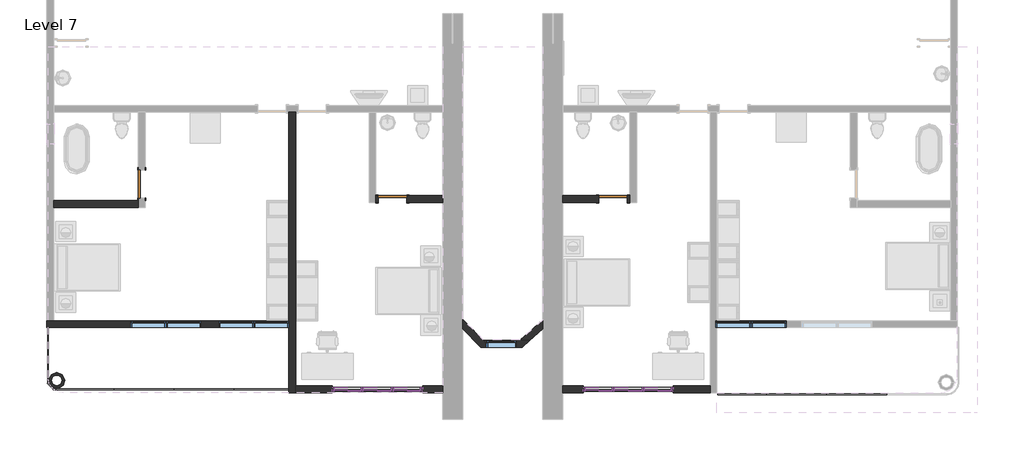
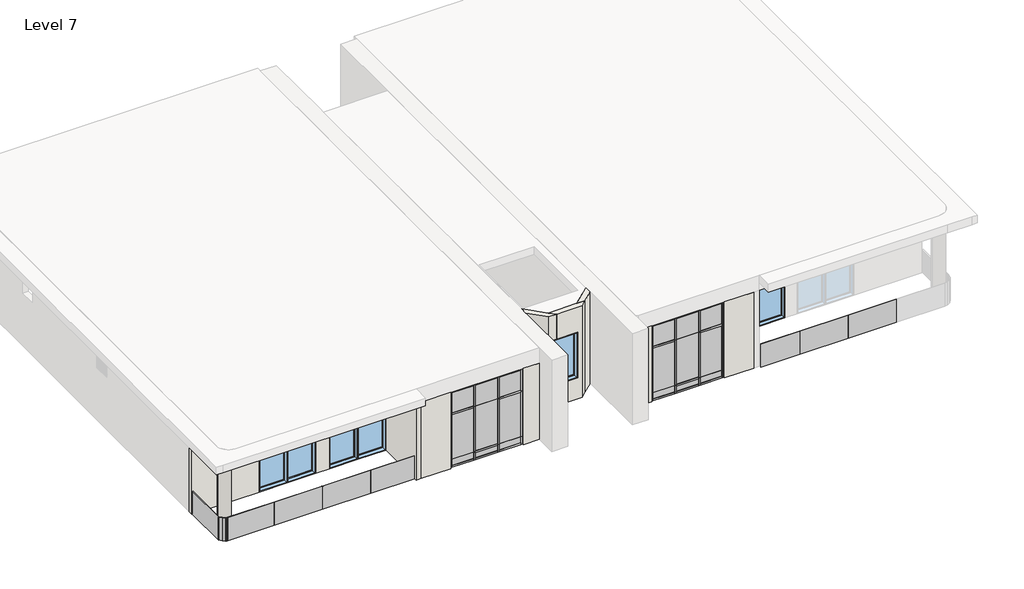
# One storey, part 1 of 3: 42 members, 30 plates, 14 walls, 7 windows, 3 doors.
"""IFC4 building model written with IfcOpenShell, lengths in millimetres."""

from ifc_helpers import new_model, si_unit, point, frame, frame_2d, origin, place, context, project, spatial, polyline, circle_curve, trimmed, segment, composite_curve, outline, extrude, faceted_brep, transform, mapped, element, save
from components import door_2703ae13, door_10fd3a06, member_c17f1be2, member_ad567e07, member_d2e7e466, member_7db1855a, member_75d1e245, member_d60e8053, member_3c3dc66a, member_2fae0574, member_410c6227, member_73c23c35, system_panel_glazed_38d54ecf, system_panel_glazed_fbb6c980, system_panel_glazed_4137532c, system_panel_glazed_6230de04, system_panel_glazed_a79f7f85, system_panel_glazed_9a5ea490, system_panel_glazed_95be5de7, system_panel_glazed_1e00a1c5, system_panel_glazed_ffe51582, system_panel_glazed_8f95e3f6, system_panel_glazed_836907cd, system_panel_glazed_688a65a2, system_panel_glazed_c1a1c740, system_panel_glazed_22bcd51f, window_9a779fa2, window_1a213a25

model = new_model("IFC4")

# Units and contexts
model_context = context("Model", 3, world=origin())
ifc_project = project(units=[si_unit("LENGTHUNIT", "METRE", prefix="MILLI")], contexts=[model_context])

# Site, building, storey
site = spatial("IfcSite", under=ifc_project)
building = spatial("IfcBuilding", under=site)
storey = spatial("IfcBuildingStorey", under=building, Name="Level 7", Elevation=21945.6)

# Doors
placement = place(None, origin())
door_shape = door_2703ae13(model_context)
element("IfcDoor", 1, ObjectType="Door-Single-Panel.0001 : 34\" x 80\"", at=placement, inside=storey, context=model_context, shape_type="MappedRepresentation", body=[
    mapped(door_shape, transform((-15759.6487704, -441.9241442, 21945.6), x_axis=(0.0, -1.0, 0.0), y_axis=(1.0, 0.0, 0.0), z_axis=(0.0, 0.0, 1.0))),
])
element("IfcDoor", 2, ObjectType="Door-Single-Panel.0001 : 34\" x 80\"", at=placement, inside=storey, context=model_context, shape_type="MappedRepresentation", body=[
    mapped(door_shape, transform((-8139.6487704, -899.1241442, 21945.6), x_axis=(-1.0, 0.0, 0.0), y_axis=(0.0, -1.0, 0.0), z_axis=(0.0, 0.0, 1.0))),
])
door_2_shape = door_10fd3a06(model_context)
element("IfcDoor", 3, ObjectType="Door-Single-Panel.0001 : 34\" x 80\"", at=placement, inside=storey, context=model_context, shape_type="MappedRepresentation", body=[
    mapped(door_2_shape, transform((-1434.0487704, -899.1241442, 21945.6), x_axis=(1.0, 0.0, 0.0), y_axis=(0.0, 1.0, 0.0), z_axis=(0.0, 0.0, 1.0))),
])

# Members
member_shape = member_c17f1be2(model_context)
element("IfcMember", 4, ObjectType="Rectangular Mullion : 2.5\" x 5\" rectangular", at=placement, inside=storey, context=model_context, shape_type="MappedRepresentation", body=[
    mapped(member_shape, transform((-9904.9487704, -6690.3241442, 24993.6), x_axis=(0.0, 0.0, 1.0), y_axis=(0.0, 1.0, 0.0), z_axis=(-1.0, 0.0, 0.0))),
])
element("IfcMember", 5, ObjectType="Rectangular Mullion : 2.5\" x 5\" rectangular", at=placement, inside=storey, context=model_context, shape_type="MappedRepresentation", body=[
    mapped(member_shape, transform((-8107.8987704, -6690.3241442, 24993.6), x_axis=(0.0, 0.0, 1.0), y_axis=(0.0, 1.0, 0.0), z_axis=(-1.0, 0.0, 0.0))),
])
element("IfcMember", 6, ObjectType="Rectangular Mullion : 2.5\" x 5\" rectangular", at=placement, inside=storey, context=model_context, shape_type="MappedRepresentation", body=[
    mapped(member_shape, transform((-2284.9487704, -6690.3241442, 24993.6), x_axis=(0.0, 0.0, 1.0), y_axis=(0.0, 1.0, 0.0), z_axis=(-1.0, 0.0, 0.0))),
])
element("IfcMember", 7, ObjectType="Rectangular Mullion : 2.5\" x 5\" rectangular", at=placement, inside=storey, context=model_context, shape_type="MappedRepresentation", body=[
    mapped(member_shape, transform((-487.8987704, -6690.3241442, 24993.6), x_axis=(0.0, 0.0, 1.0), y_axis=(0.0, 1.0, 0.0), z_axis=(-1.0, 0.0, 0.0))),
])
element("IfcMember", 8, ObjectType="Rectangular Mullion : 2.5\" x 5\" rectangular", at=placement, inside=storey, context=model_context, shape_type="MappedRepresentation", body=[
    mapped(member_shape, transform((-7288.7487704, -6690.3241442, 21945.6), x_axis=(0.0, 0.0, -1.0), y_axis=(0.0, 1.0, 0.0), z_axis=(1.0, 0.0, 0.0))),
])
element("IfcMember", 9, ObjectType="Rectangular Mullion : 2.5\" x 5\" rectangular", at=placement, inside=storey, context=model_context, shape_type="MappedRepresentation", body=[
    mapped(member_shape, transform((-9085.7987704, -6690.3241442, 21945.6), x_axis=(0.0, 0.0, -1.0), y_axis=(0.0, 1.0, 0.0), z_axis=(1.0, 0.0, 0.0))),
])
element("IfcMember", 10, ObjectType="Rectangular Mullion : 2.5\" x 5\" rectangular", at=placement, inside=storey, context=model_context, shape_type="MappedRepresentation", body=[
    mapped(member_shape, transform((331.2512296, -6690.3241442, 21945.6), x_axis=(0.0, 0.0, -1.0), y_axis=(0.0, 1.0, 0.0), z_axis=(1.0, 0.0, 0.0))),
])
element("IfcMember", 11, ObjectType="Rectangular Mullion : 2.5\" x 5\" rectangular", at=placement, inside=storey, context=model_context, shape_type="MappedRepresentation", body=[
    mapped(member_shape, transform((-1465.7987704, -6690.3241442, 21945.6), x_axis=(0.0, 0.0, -1.0), y_axis=(0.0, 1.0, 0.0), z_axis=(1.0, 0.0, 0.0))),
])
member_2_shape = member_ad567e07(model_context)
element("IfcMember", 12, ObjectType="Rectangular Mullion : 2.5\" x 5\" rectangular", at=placement, inside=storey, context=model_context, shape_type="MappedRepresentation", body=[
    mapped(member_2_shape, transform((-8107.8987704, -6690.3241442, 24079.2), x_axis=(0.0, 0.0, 1.0), y_axis=(0.0, 1.0, 0.0), z_axis=(-1.0, 0.0, 0.0))),
])
element("IfcMember", 13, ObjectType="Rectangular Mullion : 2.5\" x 5\" rectangular", at=placement, inside=storey, context=model_context, shape_type="MappedRepresentation", body=[
    mapped(member_2_shape, transform((-9904.9487704, -6690.3241442, 24079.2), x_axis=(0.0, 0.0, 1.0), y_axis=(0.0, 1.0, 0.0), z_axis=(-1.0, 0.0, 0.0))),
])
element("IfcMember", 14, ObjectType="Rectangular Mullion : 2.5\" x 5\" rectangular", at=placement, inside=storey, context=model_context, shape_type="MappedRepresentation", body=[
    mapped(member_2_shape, transform((-487.8987704, -6690.3241442, 24079.2), x_axis=(0.0, 0.0, 1.0), y_axis=(0.0, 1.0, 0.0), z_axis=(-1.0, 0.0, 0.0))),
])
element("IfcMember", 15, ObjectType="Rectangular Mullion : 2.5\" x 5\" rectangular", at=placement, inside=storey, context=model_context, shape_type="MappedRepresentation", body=[
    mapped(member_2_shape, transform((-2284.9487704, -6690.3241442, 24079.2), x_axis=(0.0, 0.0, 1.0), y_axis=(0.0, 1.0, 0.0), z_axis=(-1.0, 0.0, 0.0))),
])
member_3_shape = member_d2e7e466(model_context)
element("IfcMember", 16, ObjectType="Rectangular Mullion : 2.5\" x 5\" rectangular", at=placement, inside=storey, context=model_context, shape_type="MappedRepresentation", body=[
    mapped(member_3_shape, transform((-8171.3987704, -6690.3241442, 21945.6), x_axis=(0.0, 0.0, -1.0), y_axis=(0.0, 1.0, 0.0), z_axis=(1.0, 0.0, 0.0))),
])
element("IfcMember", 17, ObjectType="Rectangular Mullion : 2.5\" x 5\" rectangular", at=placement, inside=storey, context=model_context, shape_type="MappedRepresentation", body=[
    mapped(member_3_shape, transform((-551.3987704, -6690.3241442, 21945.6), x_axis=(0.0, 0.0, -1.0), y_axis=(0.0, 1.0, 0.0), z_axis=(1.0, 0.0, 0.0))),
])
member_4_shape = member_7db1855a(model_context)
element("IfcMember", 18, ObjectType="Rectangular Mullion : 2.5\" x 5\" rectangular", at=placement, inside=storey, context=model_context, shape_type="MappedRepresentation", body=[
    mapped(member_4_shape, transform((-9022.2987704, -6690.3241442, 22250.4), x_axis=(0.0, 0.0, 1.0), y_axis=(0.0, 1.0, 0.0), z_axis=(-1.0, 0.0, 0.0))),
])
element("IfcMember", 19, ObjectType="Rectangular Mullion : 2.5\" x 5\" rectangular", at=placement, inside=storey, context=model_context, shape_type="MappedRepresentation", body=[
    mapped(member_4_shape, transform((-1402.2987704, -6690.3241442, 22250.4), x_axis=(0.0, 0.0, 1.0), y_axis=(0.0, 1.0, 0.0), z_axis=(-1.0, 0.0, 0.0))),
])
element("IfcMember", 20, ObjectType="Rectangular Mullion : 2.5\" x 5\" rectangular", at=placement, inside=storey, context=model_context, shape_type="MappedRepresentation", body=[
    mapped(member_3_shape, transform((-9022.2987704, -6690.3241442, 24993.6), x_axis=(0.0, 0.0, 1.0), y_axis=(0.0, 1.0, 0.0), z_axis=(-1.0, 0.0, 0.0))),
])
element("IfcMember", 21, ObjectType="Rectangular Mullion : 2.5\" x 5\" rectangular", at=placement, inside=storey, context=model_context, shape_type="MappedRepresentation", body=[
    mapped(member_3_shape, transform((-1402.2987704, -6690.3241442, 24993.6), x_axis=(0.0, 0.0, 1.0), y_axis=(0.0, 1.0, 0.0), z_axis=(-1.0, 0.0, 0.0))),
])
member_5_shape = member_75d1e245(model_context)
element("IfcMember", 22, ObjectType="Rectangular Mullion : 2.5\" x 5\" rectangular", at=placement, inside=storey, context=model_context, shape_type="MappedRepresentation", body=[
    mapped(member_5_shape, transform((-8139.6487704, -6690.3241442, 21945.6), x_axis=(-1.0, 0.0, 0.0), y_axis=(0.0, 1.0, 0.0), z_axis=(0.0, 0.0, -1.0))),
])
element("IfcMember", 23, ObjectType="Rectangular Mullion : 2.5\" x 5\" rectangular", at=placement, inside=storey, context=model_context, shape_type="MappedRepresentation", body=[
    mapped(member_5_shape, transform((-9054.0487704, -6690.3241442, 21945.6), x_axis=(-1.0, 0.0, 0.0), y_axis=(0.0, 1.0, 0.0), z_axis=(0.0, 0.0, -1.0))),
])
element("IfcMember", 24, ObjectType="Rectangular Mullion : 2.5\" x 5\" rectangular", at=placement, inside=storey, context=model_context, shape_type="MappedRepresentation", body=[
    mapped(member_5_shape, transform((-519.6487704, -6690.3241442, 21945.6), x_axis=(-1.0, 0.0, 0.0), y_axis=(0.0, 1.0, 0.0), z_axis=(0.0, 0.0, -1.0))),
])
element("IfcMember", 25, ObjectType="Rectangular Mullion : 2.5\" x 5\" rectangular", at=placement, inside=storey, context=model_context, shape_type="MappedRepresentation", body=[
    mapped(member_5_shape, transform((-1434.0487704, -6690.3241442, 21945.6), x_axis=(-1.0, 0.0, 0.0), y_axis=(0.0, 1.0, 0.0), z_axis=(0.0, 0.0, -1.0))),
])
member_6_shape = member_d60e8053(model_context)
element("IfcMember", 26, ObjectType="Rectangular Mullion : 2.5\" x 5\" rectangular", at=placement, inside=storey, context=model_context, shape_type="MappedRepresentation", body=[
    mapped(member_6_shape, transform((-8139.6487704, -6690.3241442, 22250.4), x_axis=(-1.0, 0.0, 0.0), y_axis=(0.0, 1.0, 0.0), z_axis=(0.0, 0.0, -1.0))),
])
element("IfcMember", 27, ObjectType="Rectangular Mullion : 2.5\" x 5\" rectangular", at=placement, inside=storey, context=model_context, shape_type="MappedRepresentation", body=[
    mapped(member_6_shape, transform((-9054.0487704, -6690.3241442, 22250.4), x_axis=(-1.0, 0.0, 0.0), y_axis=(0.0, 1.0, 0.0), z_axis=(0.0, 0.0, -1.0))),
])
element("IfcMember", 28, ObjectType="Rectangular Mullion : 2.5\" x 5\" rectangular", at=placement, inside=storey, context=model_context, shape_type="MappedRepresentation", body=[
    mapped(member_6_shape, transform((-519.6487704, -6690.3241442, 22250.4), x_axis=(-1.0, 0.0, 0.0), y_axis=(0.0, 1.0, 0.0), z_axis=(0.0, 0.0, -1.0))),
])
element("IfcMember", 29, ObjectType="Rectangular Mullion : 2.5\" x 5\" rectangular", at=placement, inside=storey, context=model_context, shape_type="MappedRepresentation", body=[
    mapped(member_6_shape, transform((-1434.0487704, -6690.3241442, 22250.4), x_axis=(-1.0, 0.0, 0.0), y_axis=(0.0, 1.0, 0.0), z_axis=(0.0, 0.0, -1.0))),
])
member_7_shape = member_3c3dc66a(model_context)
element("IfcMember", 30, ObjectType="Rectangular Mullion : 2.5\" x 5\" rectangular", at=placement, inside=storey, context=model_context, shape_type="MappedRepresentation", body=[
    mapped(member_7_shape, transform((-9968.4487704, -6690.3241442, 21945.6), x_axis=(-1.0, 0.0, 0.0), y_axis=(0.0, 1.0, 0.0), z_axis=(0.0, 0.0, -1.0))),
])
element("IfcMember", 31, ObjectType="Rectangular Mullion : 2.5\" x 5\" rectangular", at=placement, inside=storey, context=model_context, shape_type="MappedRepresentation", body=[
    mapped(member_7_shape, transform((-2348.4487704, -6690.3241442, 21945.6), x_axis=(-1.0, 0.0, 0.0), y_axis=(0.0, 1.0, 0.0), z_axis=(0.0, 0.0, -1.0))),
])
member_8_shape = member_2fae0574(model_context)
element("IfcMember", 32, ObjectType="Rectangular Mullion : 2.5\" x 5\" rectangular", at=placement, inside=storey, context=model_context, shape_type="MappedRepresentation", body=[
    mapped(member_8_shape, transform((-9968.4487704, -6690.3241442, 22250.4), x_axis=(-1.0, 0.0, 0.0), y_axis=(0.0, 1.0, 0.0), z_axis=(0.0, 0.0, -1.0))),
])
element("IfcMember", 33, ObjectType="Rectangular Mullion : 2.5\" x 5\" rectangular", at=placement, inside=storey, context=model_context, shape_type="MappedRepresentation", body=[
    mapped(member_8_shape, transform((-2348.4487704, -6690.3241442, 22250.4), x_axis=(-1.0, 0.0, 0.0), y_axis=(0.0, 1.0, 0.0), z_axis=(0.0, 0.0, -1.0))),
])
element("IfcMember", 34, ObjectType="Rectangular Mullion : 2.5\" x 5\" rectangular", at=placement, inside=storey, context=model_context, shape_type="MappedRepresentation", body=[
    mapped(member_8_shape, transform((-7225.2487704, -6690.3241442, 24079.2), x_axis=(1.0, 0.0, 0.0), y_axis=(0.0, 1.0, 0.0), z_axis=(0.0, 0.0, 1.0))),
])
element("IfcMember", 35, ObjectType="Rectangular Mullion : 2.5\" x 5\" rectangular", at=placement, inside=storey, context=model_context, shape_type="MappedRepresentation", body=[
    mapped(member_8_shape, transform((394.7512296, -6690.3241442, 24079.2), x_axis=(1.0, 0.0, 0.0), y_axis=(0.0, 1.0, 0.0), z_axis=(0.0, 0.0, 1.0))),
])
element("IfcMember", 36, ObjectType="Rectangular Mullion : 2.5\" x 5\" rectangular", at=placement, inside=storey, context=model_context, shape_type="MappedRepresentation", body=[
    mapped(member_7_shape, transform((-7225.2487704, -6690.3241442, 22250.4), x_axis=(1.0, 0.0, 0.0), y_axis=(0.0, 1.0, 0.0), z_axis=(0.0, 0.0, 1.0))),
])
element("IfcMember", 37, ObjectType="Rectangular Mullion : 2.5\" x 5\" rectangular", at=placement, inside=storey, context=model_context, shape_type="MappedRepresentation", body=[
    mapped(member_7_shape, transform((394.7512296, -6690.3241442, 22250.4), x_axis=(1.0, 0.0, 0.0), y_axis=(0.0, 1.0, 0.0), z_axis=(0.0, 0.0, 1.0))),
])
member_9_shape = member_410c6227(model_context)
element("IfcMember", 38, ObjectType="Rectangular Mullion : 2.5\" x 5\" rectangular", at=placement, inside=storey, context=model_context, shape_type="MappedRepresentation", body=[
    mapped(member_9_shape, transform((-8139.6487704, -6690.3241442, 24079.2), x_axis=(-1.0, 0.0, 0.0), y_axis=(0.0, 1.0, 0.0), z_axis=(0.0, 0.0, -1.0))),
])
element("IfcMember", 39, ObjectType="Rectangular Mullion : 2.5\" x 5\" rectangular", at=placement, inside=storey, context=model_context, shape_type="MappedRepresentation", body=[
    mapped(member_9_shape, transform((-9054.0487704, -6690.3241442, 24079.2), x_axis=(-1.0, 0.0, 0.0), y_axis=(0.0, 1.0, 0.0), z_axis=(0.0, 0.0, -1.0))),
])
element("IfcMember", 40, ObjectType="Rectangular Mullion : 2.5\" x 5\" rectangular", at=placement, inside=storey, context=model_context, shape_type="MappedRepresentation", body=[
    mapped(member_9_shape, transform((-519.6487704, -6690.3241442, 24079.2), x_axis=(-1.0, 0.0, 0.0), y_axis=(0.0, 1.0, 0.0), z_axis=(0.0, 0.0, -1.0))),
])
element("IfcMember", 41, ObjectType="Rectangular Mullion : 2.5\" x 5\" rectangular", at=placement, inside=storey, context=model_context, shape_type="MappedRepresentation", body=[
    mapped(member_9_shape, transform((-1434.0487704, -6690.3241442, 24079.2), x_axis=(-1.0, 0.0, 0.0), y_axis=(0.0, 1.0, 0.0), z_axis=(0.0, 0.0, -1.0))),
])
member_10_shape = member_73c23c35(model_context)
element("IfcMember", 42, ObjectType="Rectangular Mullion : 2.5\" x 5\" rectangular", at=placement, inside=storey, context=model_context, shape_type="MappedRepresentation", body=[
    mapped(member_10_shape, transform((-7225.2487704, -6690.3241442, 24993.6), x_axis=(1.0, 0.0, 0.0), y_axis=(0.0, 1.0, 0.0), z_axis=(0.0, 0.0, 1.0))),
])
element("IfcMember", 43, ObjectType="Rectangular Mullion : 2.5\" x 5\" rectangular", at=placement, inside=storey, context=model_context, shape_type="MappedRepresentation", body=[
    mapped(member_10_shape, transform((394.7512296, -6690.3241442, 24993.6), x_axis=(1.0, 0.0, 0.0), y_axis=(0.0, 1.0, 0.0), z_axis=(0.0, 0.0, 1.0))),
])
element("IfcMember", 44, ObjectType="Rectangular Mullion : 2.5\" x 5\" rectangular", at=placement, inside=storey, context=model_context, shape_type="MappedRepresentation", body=[
    mapped(member_10_shape, transform((-9968.4487704, -6690.3241442, 24079.2), x_axis=(-1.0, 0.0, 0.0), y_axis=(0.0, 1.0, 0.0), z_axis=(0.0, 0.0, -1.0))),
])
element("IfcMember", 45, ObjectType="Rectangular Mullion : 2.5\" x 5\" rectangular", at=placement, inside=storey, context=model_context, shape_type="MappedRepresentation", body=[
    mapped(member_10_shape, transform((-2348.4487704, -6690.3241442, 24079.2), x_axis=(-1.0, 0.0, 0.0), y_axis=(0.0, 1.0, 0.0), z_axis=(0.0, 0.0, -1.0))),
])

# Plates
system_panel_glazed_shape = system_panel_glazed_38d54ecf(model_context)
element("IfcPlate", 46, ObjectType="System Panel : Glazed", at=placement, inside=storey, context=model_context, shape_type="MappedRepresentation", body=[
    mapped(system_panel_glazed_shape, transform((-8596.8487704, -6690.3241442, 22282.15), x_axis=(-1.0, 0.0, 0.0), y_axis=(0.0, -1.0, 0.0), z_axis=(0.0, 0.0, 1.0))),
])
element("IfcPlate", 47, ObjectType="System Panel : Glazed", at=placement, inside=storey, context=model_context, shape_type="MappedRepresentation", body=[
    mapped(system_panel_glazed_shape, transform((-976.8487704, -6690.3241442, 22282.15), x_axis=(-1.0, 0.0, 0.0), y_axis=(0.0, -1.0, 0.0), z_axis=(0.0, 0.0, 1.0))),
])
system_panel_glazed_2_shape = system_panel_glazed_fbb6c980(model_context)
element("IfcPlate", 48, ObjectType="System Panel : Glazed", at=placement, inside=storey, context=model_context, shape_type="MappedRepresentation", body=[
    mapped(system_panel_glazed_2_shape, transform((-8596.8487704, -6690.3241442, 22009.1), x_axis=(-1.0, 0.0, 0.0), y_axis=(0.0, -1.0, 0.0), z_axis=(0.0, 0.0, 1.0))),
])
element("IfcPlate", 49, ObjectType="System Panel : Glazed", at=placement, inside=storey, context=model_context, shape_type="MappedRepresentation", body=[
    mapped(system_panel_glazed_2_shape, transform((-976.8487704, -6690.3241442, 22009.1), x_axis=(-1.0, 0.0, 0.0), y_axis=(0.0, -1.0, 0.0), z_axis=(0.0, 0.0, 1.0))),
])
system_panel_glazed_3_shape = system_panel_glazed_4137532c(model_context)
element("IfcPlate", 50, ObjectType="System Panel : Glazed", at=placement, inside=storey, context=model_context, shape_type="MappedRepresentation", body=[
    mapped(system_panel_glazed_3_shape, transform((-7698.3237704, -6690.3241442, 22009.1), x_axis=(-1.0, 0.0, 0.0), y_axis=(0.0, -1.0, 0.0), z_axis=(0.0, 0.0, 1.0))),
])
element("IfcPlate", 51, ObjectType="System Panel : Glazed", at=placement, inside=storey, context=model_context, shape_type="MappedRepresentation", body=[
    mapped(system_panel_glazed_3_shape, transform((-9495.3737704, -6690.3241442, 22009.1), x_axis=(-1.0, 0.0, 0.0), y_axis=(0.0, -1.0, 0.0), z_axis=(0.0, 0.0, 1.0))),
])
element("IfcPlate", 52, ObjectType="System Panel : Glazed", at=placement, inside=storey, context=model_context, shape_type="MappedRepresentation", body=[
    mapped(system_panel_glazed_3_shape, transform((-78.3237704, -6690.3241442, 22009.1), x_axis=(-1.0, 0.0, 0.0), y_axis=(0.0, -1.0, 0.0), z_axis=(0.0, 0.0, 1.0))),
])
element("IfcPlate", 53, ObjectType="System Panel : Glazed", at=placement, inside=storey, context=model_context, shape_type="MappedRepresentation", body=[
    mapped(system_panel_glazed_3_shape, transform((-1875.3737704, -6690.3241442, 22009.1), x_axis=(-1.0, 0.0, 0.0), y_axis=(0.0, -1.0, 0.0), z_axis=(0.0, 0.0, 1.0))),
])
system_panel_glazed_4_shape = system_panel_glazed_6230de04(model_context)
element("IfcPlate", 54, ObjectType="System Panel : Glazed", at=placement, inside=storey, context=model_context, shape_type="MappedRepresentation", body=[
    mapped(system_panel_glazed_4_shape, transform((-7698.3237704, -6690.3241442, 22250.4), x_axis=(-1.0, 0.0, 0.0), y_axis=(0.0, -1.0, 0.0), z_axis=(0.0, 0.0, 1.0))),
])
element("IfcPlate", 55, ObjectType="System Panel : Glazed", at=placement, inside=storey, context=model_context, shape_type="MappedRepresentation", body=[
    mapped(system_panel_glazed_4_shape, transform((-9495.3737704, -6690.3241442, 22250.4), x_axis=(-1.0, 0.0, 0.0), y_axis=(0.0, -1.0, 0.0), z_axis=(0.0, 0.0, 1.0))),
])
element("IfcPlate", 56, ObjectType="System Panel : Glazed", at=placement, inside=storey, context=model_context, shape_type="MappedRepresentation", body=[
    mapped(system_panel_glazed_4_shape, transform((-78.3237704, -6690.3241442, 22250.4), x_axis=(-1.0, 0.0, 0.0), y_axis=(0.0, -1.0, 0.0), z_axis=(0.0, 0.0, 1.0))),
])
element("IfcPlate", 57, ObjectType="System Panel : Glazed", at=placement, inside=storey, context=model_context, shape_type="MappedRepresentation", body=[
    mapped(system_panel_glazed_4_shape, transform((-1875.3737704, -6690.3241442, 22250.4), x_axis=(-1.0, 0.0, 0.0), y_axis=(0.0, -1.0, 0.0), z_axis=(0.0, 0.0, 1.0))),
])
system_panel_glazed_5_shape = system_panel_glazed_a79f7f85(model_context)
element("IfcPlate", 58, ObjectType="System Panel : Glazed", at=placement, inside=storey, context=model_context, shape_type="MappedRepresentation", body=[
    mapped(system_panel_glazed_5_shape, transform((-7698.3237704, -6690.3241442, 24110.95), x_axis=(-1.0, 0.0, 0.0), y_axis=(0.0, -1.0, 0.0), z_axis=(0.0, 0.0, 1.0))),
])
element("IfcPlate", 59, ObjectType="System Panel : Glazed", at=placement, inside=storey, context=model_context, shape_type="MappedRepresentation", body=[
    mapped(system_panel_glazed_5_shape, transform((-9495.3737704, -6690.3241442, 24110.95), x_axis=(-1.0, 0.0, 0.0), y_axis=(0.0, -1.0, 0.0), z_axis=(0.0, 0.0, 1.0))),
])
element("IfcPlate", 60, ObjectType="System Panel : Glazed", at=placement, inside=storey, context=model_context, shape_type="MappedRepresentation", body=[
    mapped(system_panel_glazed_5_shape, transform((-78.3237704, -6690.3241442, 24110.95), x_axis=(-1.0, 0.0, 0.0), y_axis=(0.0, -1.0, 0.0), z_axis=(0.0, 0.0, 1.0))),
])
element("IfcPlate", 61, ObjectType="System Panel : Glazed", at=placement, inside=storey, context=model_context, shape_type="MappedRepresentation", body=[
    mapped(system_panel_glazed_5_shape, transform((-1875.3737704, -6690.3241442, 24110.95), x_axis=(-1.0, 0.0, 0.0), y_axis=(0.0, -1.0, 0.0), z_axis=(0.0, 0.0, 1.0))),
])
system_panel_glazed_6_shape = system_panel_glazed_9a5ea490(model_context)
element("IfcPlate", 62, ObjectType="System Panel : Glazed", at=placement, inside=storey, context=model_context, shape_type="MappedRepresentation", body=[
    mapped(system_panel_glazed_6_shape, transform((-8596.8487704, -6690.3241442, 24079.2), x_axis=(-1.0, 0.0, 0.0), y_axis=(0.0, -1.0, 0.0), z_axis=(0.0, 0.0, 1.0))),
])
element("IfcPlate", 63, ObjectType="System Panel : Glazed", at=placement, inside=storey, context=model_context, shape_type="MappedRepresentation", body=[
    mapped(system_panel_glazed_6_shape, transform((-976.8487704, -6690.3241442, 24079.2), x_axis=(-1.0, 0.0, 0.0), y_axis=(0.0, -1.0, 0.0), z_axis=(0.0, 0.0, 1.0))),
])
system_panel_glazed_7_shape = system_panel_glazed_95be5de7(model_context)
element("IfcPlate", 64, ObjectType="System Panel : Glazed", at=placement, inside=storey, context=model_context, shape_type="MappedRepresentation", body=[
    mapped(system_panel_glazed_7_shape, transform((-15700.8805745, -6723.6923401, 21945.6), x_axis=(1.0, 0.0, 0.0), y_axis=(0.0, 1.0, 0.0), z_axis=(0.0, 0.0, 1.0))),
])
element("IfcPlate", 65, ObjectType="System Panel : Glazed", at=placement, inside=storey, context=model_context, shape_type="MappedRepresentation", body=[
    mapped(system_panel_glazed_7_shape, transform((-13872.0805745, -6723.6923401, 21945.6), x_axis=(1.0, 0.0, 0.0), y_axis=(0.0, 1.0, 0.0), z_axis=(0.0, 0.0, 1.0))),
])
element("IfcPlate", 66, ObjectType="System Panel : Glazed", at=placement, inside=storey, context=model_context, shape_type="MappedRepresentation", body=[
    mapped(system_panel_glazed_7_shape, transform((5964.2620092, -6810.4133646, 21945.6), x_axis=(-1.0, 0.0, 0.0), y_axis=(0.0, -1.0, 0.0), z_axis=(0.0, 0.0, 1.0))),
])
element("IfcPlate", 67, ObjectType="System Panel : Glazed", at=placement, inside=storey, context=model_context, shape_type="MappedRepresentation", body=[
    mapped(system_panel_glazed_7_shape, transform((4135.4620092, -6810.4133646, 21945.6), x_axis=(-1.0, 0.0, 0.0), y_axis=(0.0, -1.0, 0.0), z_axis=(0.0, 0.0, 1.0))),
])
system_panel_glazed_8_shape = system_panel_glazed_1e00a1c5(model_context)
element("IfcPlate", 68, ObjectType="System Panel : Glazed", at=placement, inside=storey, context=model_context, shape_type="MappedRepresentation", body=[
    mapped(system_panel_glazed_8_shape, transform((2484.4620092, -6810.4133646, 21945.6), x_axis=(-1.0, 0.0, 0.0), y_axis=(0.0, -1.0, 0.0), z_axis=(0.0, 0.0, 1.0))),
])
system_panel_glazed_9_shape = system_panel_glazed_ffe51582(model_context)
element("IfcPlate", 69, ObjectType="System Panel : Glazed", at=placement, inside=storey, context=model_context, shape_type="MappedRepresentation", body=[
    mapped(system_panel_glazed_9_shape, transform((-18445.6213429, -6722.1515718, 21945.6), x_axis=(0.7071067811865462, -0.7071067811865488, 0.0), y_axis=(0.7071067811865488, 0.7071067811865462, 0.0), z_axis=(0.0, 0.0, 1.0))),
])
system_panel_glazed_10_shape = system_panel_glazed_8f95e3f6(model_context)
element("IfcPlate", 70, ObjectType="System Panel : Glazed", at=placement, inside=storey, context=model_context, shape_type="MappedRepresentation", body=[
    mapped(system_panel_glazed_10_shape, transform((-18642.5487704, -5667.9741442, 21945.6), x_axis=(0.0, -1.0, 0.0), y_axis=(1.0, 0.0, 0.0), z_axis=(0.0, 0.0, 1.0))),
])
system_panel_glazed_11_shape = system_panel_glazed_836907cd(model_context)
element("IfcPlate", 71, ObjectType="System Panel : Glazed", at=placement, inside=storey, context=model_context, shape_type="MappedRepresentation", body=[
    mapped(system_panel_glazed_11_shape, transform((-18412.3305745, -6723.6923401, 21945.6), x_axis=(1.0, 0.0, 0.0), y_axis=(0.0, 1.0, 0.0), z_axis=(0.0, 0.0, 1.0))),
])
system_panel_glazed_12_shape = system_panel_glazed_688a65a2(model_context)
element("IfcPlate", 72, ObjectType="System Panel : Glazed", at=placement, inside=storey, context=model_context, shape_type="MappedRepresentation", body=[
    mapped(system_panel_glazed_12_shape, transform((-12123.4646725, -6723.6923401, 21945.6), x_axis=(1.0, 0.0, 0.0), y_axis=(0.0, 1.0, 0.0), z_axis=(0.0, 0.0, 1.0))),
])
system_panel_glazed_13_shape = system_panel_glazed_c1a1c740(model_context)
element("IfcPlate", 73, ObjectType="System Panel : Glazed", at=placement, inside=storey, context=model_context, shape_type="MappedRepresentation", body=[
    mapped(system_panel_glazed_13_shape, transform((-17497.9305745, -6723.6923401, 21945.6), x_axis=(1.0, 0.0, 0.0), y_axis=(0.0, 1.0, 0.0), z_axis=(0.0, 0.0, 1.0))),
])
system_panel_glazed_14_shape = system_panel_glazed_22bcd51f(model_context)
element("IfcPlate", 74, ObjectType="System Panel : Glazed", at=placement, inside=storey, context=model_context, shape_type="MappedRepresentation", body=[
    mapped(system_panel_glazed_14_shape, transform((-18593.7021056, -6574.070809, 21945.6), x_axis=(0.7071067811865462, -0.7071067811865488, 0.0), y_axis=(0.7071067811865488, 0.7071067811865462, 0.0), z_axis=(0.0, 0.0, 1.0))),
])
element("IfcPlate", 75, ObjectType="System Panel : Glazed", at=placement, inside=storey, context=model_context, shape_type="MappedRepresentation", body=[
    mapped(system_panel_glazed_14_shape, transform((-18496.0087761, -6671.7641386, 21945.6), x_axis=(0.7071067811865462, -0.7071067811865488, 0.0), y_axis=(0.7071067811865488, 0.7071067811865462, 0.0), z_axis=(0.0, 0.0, 1.0))),
])

# Walls
element("IfcWall", 76, ObjectType="Generic - 3\" green 2", at=placement, inside=storey, context=model_context, shape_type="SweptSolid", body=[
    extrude(outline(composite_curve([segment(polyline([(-18512.3737704, -6418.8616442), (-18588.5737704, -6418.8616442)]), True, "CONTINUOUS"), segment(trimmed(circle_curve(frame_2d((-18347.2737704, -6418.8616442)), 241.3), [point((-18588.5737704, -6418.8616442))], [point((-18105.9737704, -6418.8616442))], False, "CARTESIAN"), True, "CONTINUOUS"), segment(polyline([(-18105.9737704, -6418.8616442), (-18182.1737704, -6418.8616442)]), True, "CONTINUOUS"), segment(trimmed(circle_curve(frame_2d((-18347.2737704, -6418.8616442)), 165.1), [point((-18182.1737704, -6418.8616442))], [point((-18512.3737704, -6418.8616442))], True, "CARTESIAN"), True, "CONTINUOUS")], self_intersect=False)), frame((0.0, 0.0, 21945.6), z_axis=(0.0, 0.0, 1.0), x_axis=(1.0, 0.0, 0.0)), (0.0, 0.0, 1.0), 3048.0),
])
element("IfcWall", 77, ObjectType="Generic - 3\" green 2", at=placement, inside=storey, context=model_context, shape_type="SweptSolid", body=[
    extrude(outline(composite_curve([segment(polyline([(-18182.1737704, -6418.8616442), (-18105.9737704, -6418.8616442)]), True, "CONTINUOUS"), segment(trimmed(circle_curve(frame_2d((-18347.2737704, -6418.8616442)), 241.3), [point((-18105.9737704, -6418.8616442))], [point((-18588.5737704, -6418.8616442))], False, "CARTESIAN"), True, "CONTINUOUS"), segment(polyline([(-18588.5737704, -6418.8616442), (-18512.3737704, -6418.8616442)]), True, "CONTINUOUS"), segment(trimmed(circle_curve(frame_2d((-18347.2737704, -6418.8616442)), 165.1), [point((-18512.3737704, -6418.8616442))], [point((-18182.1737704, -6418.8616442))], True, "CARTESIAN"), True, "CONTINUOUS")], self_intersect=False)), frame((0.0, 0.0, 21945.6), z_axis=(0.0, 0.0, 1.0), x_axis=(1.0, 0.0, 0.0)), (0.0, 0.0, 1.0), 3048.0),
])
element("IfcWall", 78, ObjectType="Generic - 8\" cream", at=placement, inside=storey, context=model_context, shape_type="Brep", body=[
    faceted_brep([(-11289.2487704, 1742.4758558, 21945.6), (-11289.2487704, -6791.9241442, 21945.6), (-11289.2487704, -6791.9241442, 24993.6), (-11289.2487704, -4810.7241442, 24993.6), (-11289.2487704, -4607.5241442, 24993.6), (-11289.2487704, 1742.4758558, 24993.6), (-11086.0487704, 1742.4758558, 21945.6), (-11086.0487704, 1742.4758558, 24993.6), (-11086.0487704, -6588.7241442, 24993.6), (-11086.0487704, -6791.9241442, 24993.6), (-11086.0487704, -6791.9241442, 21945.6), (-11086.0487704, -6588.7241442, 21945.6)], [[[0, 1, 2, 3, 4, 5]], [[6, 7, 8, 9, 10, 11]], [[1, 0, 6, 11, 10]], [[5, 4, 3, 2, 9, 8, 7]], [[0, 5, 7, 6]], [[2, 1, 10, 9]]]),
])
element("IfcWall", 79, ObjectType="Generic - 8\" cream", at=placement, inside=storey, context=model_context, shape_type="SweptSolid", body=[
    extrude(outline(polyline([(-18439.3487704, -949.9241442), (-15861.2487704, -949.9241442), (-15861.2487704, -1153.1241442), (-18439.3487704, -1153.1241442), (-18439.3487704, -949.9241442)])), frame((0.0, 0.0, 21945.6), z_axis=(0.0, 0.0, 1.0), x_axis=(1.0, 0.0, 0.0)), (0.0, 0.0, 1.0), 3048.0),
])
element("IfcWall", 80, ObjectType="Generic - 8\" cream", at=placement, inside=storey, context=model_context, shape_type="SweptSolid", body=[
    extrude(outline(polyline([(24993.6, -6615.6487704), (24993.6, -8647.6487704), (21945.6, -8647.6487704), (21945.6, -8571.4487704), (23977.6, -8571.4487704), (23977.6, -7707.8487704), (21945.6, -7707.8487704), (21945.6, -6615.6487704), (24993.6, -6615.6487704)])), frame((0.0, -1000.7241442, 0.0), z_axis=(0.0, 1.0, 0.0), x_axis=(0.0, 0.0, 1.0)), (0.0, 0.0, 1.0), 203.2),
])
element("IfcWall", 81, ObjectType="Generic - 8\" cream", at=placement, inside=storey, context=model_context, shape_type="Brep", body=[
    faceted_brep([(-18642.5487704, -4607.5241442, 24993.6), (-18439.3487704, -4607.5241442, 24993.6), (-11289.2487704, -4607.5241442, 24993.6), (-11289.2487704, -4607.5241442, 24688.8), (-13422.8487704, -4607.5241442, 24688.8), (-13422.8487704, -4607.5241442, 21945.6), (-13956.2487704, -4607.5241442, 21945.6), (-13956.2487704, -4607.5241442, 24688.8), (-16089.8487704, -4607.5241442, 24688.8), (-16089.8487704, -4607.5241442, 21945.6), (-18439.3487704, -4607.5241442, 21945.6), (-18642.5487704, -4607.5241442, 21945.6), (-11289.2487704, -4810.7241442, 24993.6), (-18642.5487704, -4810.7241442, 24993.6), (-18642.5487704, -4810.7241442, 21945.6), (-16089.8487704, -4810.7241442, 21945.6), (-16089.8487704, -4810.7241442, 24688.8), (-13956.2487704, -4810.7241442, 24688.8), (-13956.2487704, -4810.7241442, 21945.6), (-13422.8487704, -4810.7241442, 21945.6), (-13422.8487704, -4810.7241442, 24688.8), (-11289.2487704, -4810.7241442, 24688.8)], [[[0, 1, 2, 3, 4, 5, 6, 7, 8, 9, 10, 11]], [[12, 13, 14, 15, 16, 17, 18, 19, 20, 21]], [[14, 11, 10, 9, 15]], [[5, 19, 18, 6]], [[2, 1, 0, 13, 12]], [[2, 12, 21, 3]], [[0, 11, 14, 13]], [[3, 21, 20, 4]], [[4, 20, 19, 5]], [[17, 7, 6, 18]], [[7, 17, 16, 8]], [[8, 16, 15, 9]]]),
])
element("IfcWall", 82, ObjectType="Generic - 8\" cream", at=placement, inside=storey, context=model_context, shape_type="SweptSolid", body=[
    extrude(outline(polyline([(24993.6, -926.0487704), (24993.6, -2958.0487704), (21945.6, -2958.0487704), (21945.6, -1865.8487704), (23977.6, -1865.8487704), (23977.6, -1002.2487704), (21945.6, -1002.2487704), (21945.6, -926.0487704), (24993.6, -926.0487704)])), frame((0.0, -1000.7241442, 0.0), z_axis=(0.0, 1.0, 0.0), x_axis=(0.0, 0.0, 1.0)), (0.0, 0.0, 1.0), 203.2),
])
element("IfcWall", 83, ObjectType="Generic - 8\" cream", at=placement, inside=storey, context=model_context, shape_type="SweptSolid", body=[
    extrude(outline(polyline([(394.7512296, -6588.7241442), (1512.3512296, -6588.7241442), (1512.3512296, -6791.9241442), (394.7512296, -6791.9241442), (394.7512296, -6588.7241442)])), frame((0.0, 0.0, 21945.6), z_axis=(0.0, 0.0, 1.0), x_axis=(1.0, 0.0, 0.0)), (0.0, 0.0, 1.0), 3048.0),
])
element("IfcWall", 84, ObjectType="Generic - 8\" cream", at=placement, inside=storey, context=model_context, shape_type="SweptSolid", body=[
    extrude(outline(polyline([(-2348.4487704, -6791.9241442), (-2958.0487704, -6791.9241442), (-2958.0487704, -6588.7241442), (-2348.4487704, -6588.7241442), (-2348.4487704, -6791.9241442)])), frame((0.0, 0.0, 21945.6), z_axis=(0.0, 0.0, 1.0), x_axis=(1.0, 0.0, 0.0)), (0.0, 0.0, 1.0), 3048.0),
])
element("IfcWall", 85, ObjectType="Generic - 8\" cream", at=placement, inside=storey, context=model_context, shape_type="SweptSolid", body=[
    extrude(outline(polyline([(-9968.4487704, -6791.9241442), (-11086.0487704, -6791.9241442), (-11086.0487704, -6588.7241442), (-9968.4487704, -6588.7241442), (-9968.4487704, -6791.9241442)])), frame((0.0, 0.0, 21945.6), z_axis=(0.0, 0.0, 1.0), x_axis=(1.0, 0.0, 0.0)), (0.0, 0.0, 1.0), 3048.0),
])
element("IfcWall", 86, ObjectType="Generic - 8\" cream", at=placement, inside=storey, context=model_context, shape_type="SweptSolid", body=[
    extrude(outline(polyline([(-7225.2487704, -6588.7241442), (-6615.6487704, -6588.7241442), (-6615.6487704, -6791.9241442), (-7225.2487704, -6791.9241442), (-7225.2487704, -6588.7241442)])), frame((0.0, 0.0, 21945.6), z_axis=(0.0, 0.0, 1.0), x_axis=(1.0, 0.0, 0.0)), (0.0, 0.0, 1.0), 3048.0),
])
element("IfcWall", 87, ObjectType="Generic - 8\" green", at=placement, inside=storey, context=model_context, shape_type="Brep", body=[
    faceted_brep([(-6006.0487704, -4852.8082422, 21945.6), (-5452.3544276, -5406.502585, 21945.6), (-5452.3544276, -5406.502585, 25603.2), (-6006.0487704, -4852.8082422, 25603.2), (-5164.9862318, -5406.502585, 21945.6), (-5368.1862318, -5203.302585, 21945.6), (-6006.0487704, -4565.4400463, 21945.6), (-6006.0487704, -4565.4400463, 25603.2), (-5368.1862318, -5203.302585, 25603.2), (-5164.9862318, -5406.502585, 25603.2), (-5164.9862318, -5406.502585, 24612.6), (-5283.1401401, -5288.3486766, 24612.6), (-5283.1401401, -5288.3486766, 22783.8), (-5164.9862318, -5406.502585, 22783.8), (-5283.1401401, -5406.502585, 22783.8), (-5283.1401401, -5406.502585, 24612.6)], [[[0, 1, 2, 3]], [[4, 5, 6, 7, 8, 9, 10, 11, 12, 13]], [[1, 0, 6, 5, 4]], [[3, 2, 9, 8, 7]], [[0, 3, 7, 6]], [[2, 1, 4, 13, 14, 15, 10, 9]], [[12, 14, 13]], [[14, 12, 11, 15]], [[15, 11, 10]]]),
])
element("IfcWall", 88, ObjectType="Generic - 8\" green", at=placement, inside=storey, context=model_context, shape_type="Brep", body=[
    faceted_brep([(-5164.9862318, -5406.502585, 21945.6), (-4196.9843712, -5406.502585, 21945.6), (-4196.9843712, -5406.502585, 25603.2), (-5164.9862318, -5406.502585, 25603.2), (-5164.9862318, -5406.502585, 24612.6), (-4368.7401401, -5406.502585, 24612.6), (-4368.7401401, -5406.502585, 22783.8), (-5164.9862318, -5406.502585, 22783.8), (-3969.1320774, -5203.302585, 21945.6), (-4274.4301413, -5203.302585, 21945.6), (-5368.1862318, -5203.302585, 21945.6), (-5368.1862318, -5203.302585, 25603.2), (-4274.4301413, -5203.302585, 25603.2), (-3969.1320774, -5203.302585, 25603.2), (-4368.7401401, -5203.302585, 22783.8), (-4368.7401401, -5203.302585, 24612.6), (-5283.1401401, -5203.302585, 24612.6), (-5283.1401401, -5203.302585, 22783.8), (-5283.1401401, -5288.3486766, 22783.8), (-5283.1401401, -5288.3486766, 24612.6)], [[[0, 1, 2, 3, 4, 5, 6, 7]], [[8, 9, 10, 11, 12, 13], [14, 15, 16, 17]], [[1, 0, 10, 9, 8]], [[3, 2, 13, 12, 11]], [[3, 11, 10, 0, 7, 18, 19, 4]], [[2, 1, 8, 13]], [[5, 15, 14, 6]], [[6, 14, 17, 18, 7]], [[18, 17, 16, 19]], [[15, 5, 4, 19, 16]]]),
])
element("IfcWall", 89, ObjectType="Generic - 8\" green", at=placement, inside=storey, context=model_context, shape_type="SweptSolid", body=[
    extrude(outline(polyline([(-3567.6487704, -4845.2574382), (-3969.1320774, -5203.302585), (-4274.4301413, -5203.302585), (-3567.6487704, -4572.9908503), (-3567.6487704, -4845.2574382)])), frame((0.0, 0.0, 21945.6), z_axis=(0.0, 0.0, 1.0), x_axis=(1.0, 0.0, 0.0)), (0.0, 0.0, 1.0), 3657.6),
])

# Windows
window_shape = window_9a779fa2(model_context)
element("IfcWindow", 90, ObjectType="Fixed : 36\" x 72\"", at=placement, inside=storey, context=model_context, shape_type="MappedRepresentation", body=[
    mapped(window_shape, transform((-4787.8401401, -5304.902585, 22479.0), x_axis=(1.0, 0.0, 0.0), y_axis=(0.0, 1.0, 0.0), z_axis=(0.0, 0.0, 1.0))),
])
window_2_shape = window_1a213a25(model_context)
element("IfcWindow", 91, ObjectType="Fixed : 36\" x 72\" 2", at=placement, inside=storey, context=model_context, shape_type="MappedRepresentation", body=[
    mapped(window_2_shape, transform((-11784.5487704, -4709.1241442, 21640.8), x_axis=(1.0, 0.0, 0.0), y_axis=(0.0, 1.0, 0.0), z_axis=(0.0, 0.0, 1.0))),
])
element("IfcWindow", 92, ObjectType="Fixed : 36\" x 72\" 2", at=placement, inside=storey, context=model_context, shape_type="MappedRepresentation", body=[
    mapped(window_2_shape, transform((-12851.3487704, -4709.1241442, 21640.8), x_axis=(1.0, 0.0, 0.0), y_axis=(0.0, 1.0, 0.0), z_axis=(0.0, 0.0, 1.0))),
])
element("IfcWindow", 93, ObjectType="Fixed : 36\" x 72\" 2", at=placement, inside=storey, context=model_context, shape_type="MappedRepresentation", body=[
    mapped(window_2_shape, transform((-14451.5487704, -4709.1241442, 21640.8), x_axis=(1.0, 0.0, 0.0), y_axis=(0.0, 1.0, 0.0), z_axis=(0.0, 0.0, 1.0))),
])
element("IfcWindow", 94, ObjectType="Fixed : 36\" x 72\" 2", at=placement, inside=storey, context=model_context, shape_type="MappedRepresentation", body=[
    mapped(window_2_shape, transform((-15518.3487704, -4709.1241442, 21640.8), x_axis=(1.0, 0.0, 0.0), y_axis=(0.0, 1.0, 0.0), z_axis=(0.0, 0.0, 1.0))),
])
element("IfcWindow", 95, ObjectType="Fixed : 36\" x 72\" 2", at=placement, inside=storey, context=model_context, shape_type="MappedRepresentation", body=[
    mapped(window_2_shape, transform((2261.6512296, -4709.1241442, 21640.8), x_axis=(1.0, 0.0, 0.0), y_axis=(0.0, 1.0, 0.0), z_axis=(0.0, 0.0, 1.0))),
])
element("IfcWindow", 96, ObjectType="Fixed : 36\" x 72\" 2", at=placement, inside=storey, context=model_context, shape_type="MappedRepresentation", body=[
    mapped(window_2_shape, transform((3337.9762296, -4709.1241442, 21640.8), x_axis=(1.0, 0.0, 0.0), y_axis=(0.0, 1.0, 0.0), z_axis=(0.0, 0.0, 1.0))),
])

save(model, "model.ifc")

# Revit data of these elements
# Type "Door-Single-Panel.0001 : 34\" x 80\""
#   Type Mark = "9"
#   Construction Type Id = "DOOR"
#   Assembly Code = "C1020300"
#   Analytic Construction = "Wooden"
#   Thickness = 0' - 2"
#   Thermal Resistance (R) = 0.455703 (m²·K)/W
#   Swing Angle [instance default] = 90.00°
#   Heat Transfer Coefficient (U) = 2.19465 W/(m²·K)
#   Height = 6' - 8"
#   Trim Projection Ext = 0' - 1"
#   Trim Projection Int = 0' - 1"
#   Trim Width = 0' - 3"
#   Width = 2' - 10"
#   Panel Material = Wood - Birch - Solid Stained Light Low Gloss
#   Trim Material = Paint - Sienna
#   Visual Light Transmittance = 0
#   Solar Heat Gain Coefficient = 0
#   Function = (empty or 0)
#   Wall Closure = (empty or 0)
# Type "Rectangular Mullion : 2.5\" x 5\" rectangular"
#   built-in parameter 1007304 = 0.416667 (stored number, unit not read)
#   built-in parameter 1007301 = 0.104167 (stored number, unit not read)
#   built-in parameter 1007300 = 0.104167 (stored number, unit not read)
# Type "System Panel : Glazed"
#   Construction Type Id = "GSP4R"
#   Analytic Construction = "1/8 in Pilkington single glazing"
#   Visual Light Transmittance = 0.9
#   Solar Heat Gain Coefficient = 0.86
#   Heat Transfer Coefficient (U) = 6.7069 W/(m²·K)
# Type "Generic - 3\" green 2"
#   Assembly Code = "B2010"
#   Width = 0' - 3"
#   Layers, outside or top first: 0' - 3" "Damp-proofing" (function 1)
# Type "Generic - 8\" cream"
#   Assembly Code = "B2010"
#   Width = 0' - 8"
#   Layers, outside or top first: 0' - 8" "Parking Stripe" (function 1)
# Type "Generic - 8\" green"
#   Assembly Code = "B2010"
#   Width = 0' - 8"
#   Layers, outside or top first: 0' - 8" "Damp-proofing" (function 1)
# Type "Fixed : 36\" x 72\""
#   Type Mark = "9"
#   Construction Type Id = "GSP4R"
#   Assembly Code = "B2020100"
#   Analytic Construction = "1/8 in Pilkington single glazing"
#   Visual Light Transmittance = 0.9
#   Solar Heat Gain Coefficient = 0.78
#   Heat Transfer Coefficient (U) = 3.6886 W/(m²·K)
#   Height = 6' - 0"
#   Default Sill Height = 1' - 0"
#   Width = 3' - 0"
#   Window Inset = 0' - 0 3/4"
#   Glass Pane Material = Glass
#   Sash Material = Iron, Ductile
#   Wall Closure = (empty or 0)
# Type "Fixed : 36\" x 72\" 2"
#   Type Mark = "29"
#   Construction Type Id = "GSP4R"
#   Assembly Code = "B2020100"
#   Analytic Construction = "1/8 in Pilkington single glazing"
#   Visual Light Transmittance = 0.9
#   Solar Heat Gain Coefficient = 0.78
#   Heat Transfer Coefficient (U) = 3.6886 W/(m²·K)
#   Height = 9' - 0"
#   Default Sill Height = 1' - 0"
#   Width = 3' - 6"
#   Window Inset = 0' - 0 3/4"
#   Glass Pane Material = Glass
#   Sash Material = Iron, Ductile
#   Wall Closure = (empty or 0)
# Elements 1, 2, 3 (IfcDoor, "Door-Single-Panel.0001 : 34\" x 80\"")
#   Swing Angle = 90.00°
#   Phase Created = New Construction
#   Materials on its faces: "Paint - Sienna", "Wood - Birch - Solid Stained Light Low Gloss"
# Elements 4, 5, 6, 7, 8, 9, 10, 11, 12, 13, 14, 15, 16, 17, 18, 19, 20, 21, 22, 23, 24, 25, 26, 27, 28, 29, 30, 31, 32, 33, 34, 35, 36, 37, 38, 39, 40, 41, 42, 43, 44, 45 (IfcMember, "Rectangular Mullion : 2.5\" x 5\" rectangular")
#   Phase Created = New Construction
#   Materials on its faces: "Iron, Ductile"
# Elements 46, 47, 48, 49, 50, 51, 52, 53, 54, 55, 56, 57, 58, 59, 60, 61, 62, 63, 64, 65, 66, 67, 68, 69, 70, 71, 72, 73, 74, 75 (IfcPlate, "System Panel : Glazed")
#   Phase Created = New Construction
#   Materials on its faces: "Glass"
# Elements 76, 77 (IfcWall, "Generic - 3\" green 2")
#   Top Offset = 0' - 0"
#   Base Offset = 0' - 0"
#   Unconnected Height = 10' - 0"
#   wall height = 10' - 0"
#   Phase Created = New Construction
#   Materials on its faces: "Damp-proofing"
# Elements 78, 79, 80, 81, 82, 83, 84, 85, 86 (IfcWall, "Generic - 8\" cream")
#   Top Offset = 0' - 0"
#   Base Offset = 0' - 0"
#   Unconnected Height = 10' - 0"
#   wall height = 10' - 0"
#   Phase Created = New Construction
#   Base Constraint = Level 7
#   Materials on its faces: "Parking Stripe"
# Elements 87, 88, 89 (IfcWall, "Generic - 8\" green")
#   Top Offset = 0' - 0"
#   Base Offset = 0' - 0"
#   Unconnected Height = 12' - 0"
#   wall height = 12' - 0"
#   Phase Created = New Construction
#   Base Constraint = Level 7
#   Materials on its faces: "Damp-proofing"
# Element 90 (IfcWindow, "Fixed : 36\" x 72\"")
#   Mark = "169"
#   Phase Created = New Construction
#   Materials on its faces: "Iron, Ductile", "Glass"
# Element 91 (IfcWindow, "Fixed : 36\" x 72\" 2")
#   Mark = "170"
#   Phase Created = New Construction
#   Materials on its faces: "Iron, Ductile", "Glass"
# Element 92 (IfcWindow, "Fixed : 36\" x 72\" 2")
#   Mark = "171"
#   Phase Created = New Construction
#   Materials on its faces: "Iron, Ductile", "Glass"
# Element 93 (IfcWindow, "Fixed : 36\" x 72\" 2")
#   Mark = "172"
#   Phase Created = New Construction
#   Materials on its faces: "Iron, Ductile", "Glass"
# Element 94 (IfcWindow, "Fixed : 36\" x 72\" 2")
#   Mark = "173"
#   Phase Created = New Construction
#   Materials on its faces: "Iron, Ductile", "Glass"
# Element 95 (IfcWindow, "Fixed : 36\" x 72\" 2")
#   Mark = "174"
#   Phase Created = New Construction
#   Materials on its faces: "Iron, Ductile", "Glass"
# Element 96 (IfcWindow, "Fixed : 36\" x 72\" 2")
#   Mark = "175"
#   Phase Created = New Construction
#   Materials on its faces: "Iron, Ductile", "Glass"
# Materials
#   "Wood - Birch - Solid Stained Light Low Gloss": class "Wood", colour RGB 210 159 95, transparency 0, Cost = 0
#   "Paint - Sienna": colour RGB 118 70 51, transparency 0, Cost = 0
#   "Damp-proofing": class "Generic", colour RGB 127 127 127, transparency 0, Description = "Damp-proofing", Cost = 0
#   "Parking Stripe": class "Paint", colour RGB 250 250 91, transparency 0, Cost = 0
#   "Glass": class "Glass", colour RGB 0 128 192, transparency 0.75, Description = "Soda Lime Glass", Cost = 0
#   "Iron, Ductile": class "Metal", colour RGB 0 0 0, transparency 0, Description = "Ductile cast iron", Cost = 0
